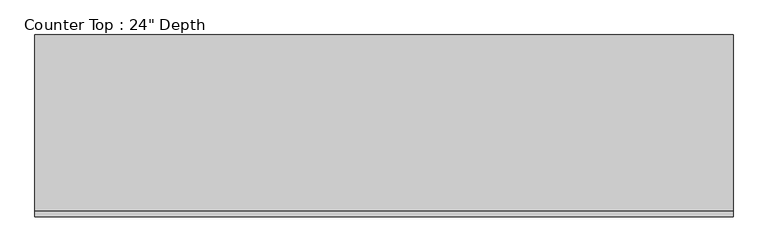
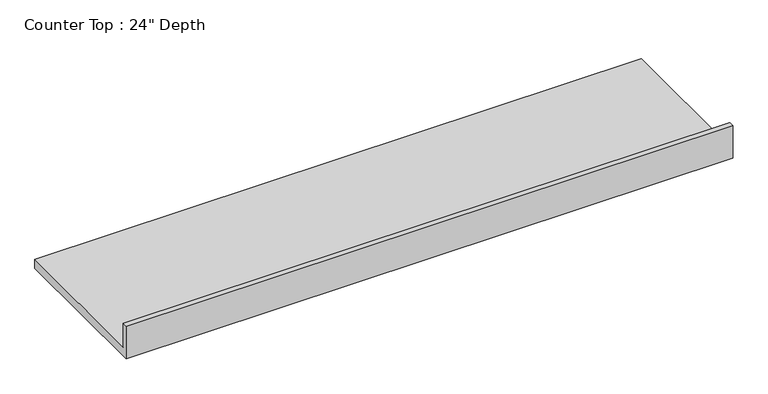
"""IFC4 building model written with IfcOpenShell, lengths in millimetres: furniture geometry."""

from ifc_helpers import new_model, si_unit, frame, origin, place, context, project, spatial, polyline, outline, extrude, source, transform, mapped, element, save


def furniture_78fcf777(model_context):
    return source(origin(), model_context, "Body", "SweptSolid", [
        extrude(outline(polyline([(0.0, 1016.0), (19.05, 1016.0), (19.05, 914.4), (635.0, 914.4), (635.0, 876.3), (0.0, 876.3), (0.0, 1016.0)])), frame((-1200.4622951, 0.0, 0.0), z_axis=(1.0, 0.0, 0.0), x_axis=(0.0, 1.0, 0.0)), (0.0, 0.0, 1.0), 2438.4),
    ])


if __name__ == "__main__":
    model = new_model("IFC4")
    model_context = context("Model", 3, world=origin())
    ifc_project = project(units=[si_unit("LENGTHUNIT", "METRE", prefix="MILLI")], contexts=[model_context])
    site = spatial("IfcSite", under=ifc_project)
    building = spatial("IfcBuilding", under=site)
    placement = place(None, origin())
    furniture_shape = furniture_78fcf777(model_context)
    element("IfcFurniture", 1, ObjectType="Counter Top : 24\" Depth", at=placement, inside=building, context=model_context, shape_type="MappedRepresentation", body=[
        mapped(furniture_shape, transform((0.0, 0.0, 0.0), x_axis=(1.0, 0.0, 0.0), y_axis=(0.0, 1.0, 0.0), z_axis=(0.0, 0.0, 1.0))),
    ])
    save(model, "model.ifc")

# Revit data of these elements
# Type "Counter Top : 24\" Depth"
#   Assembly Code = "C1030400"
#   Counter Thickness = 0' - 1 1/2"
#   Depth = 2' - 1"
#   Height = 3' - 0"
#   Length [instance default] = 8' - 0"
#   Counter Top Material = none
#   Default Elevation = 0
# Element 1 (IfcFurniture, "Counter Top : 24\" Depth")
#   Materials on its faces: "Counter Top"
# Materials
#   "Counter Top": class "Wood", colour RGB 226 177 128, transparency 0
